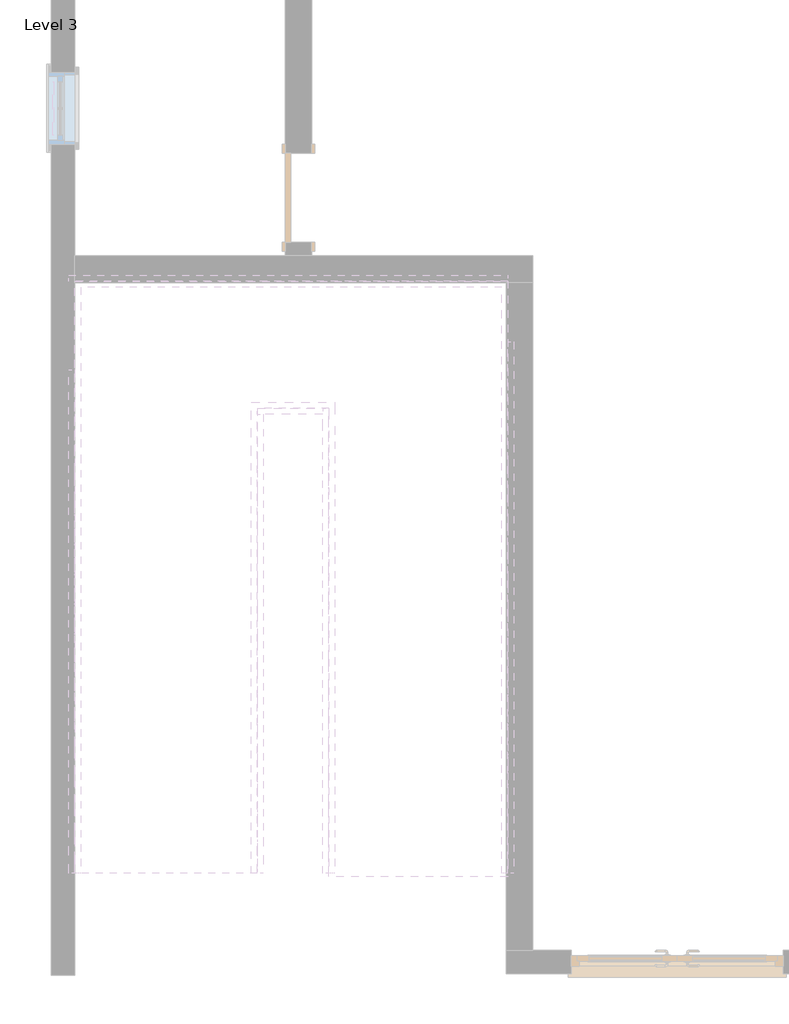
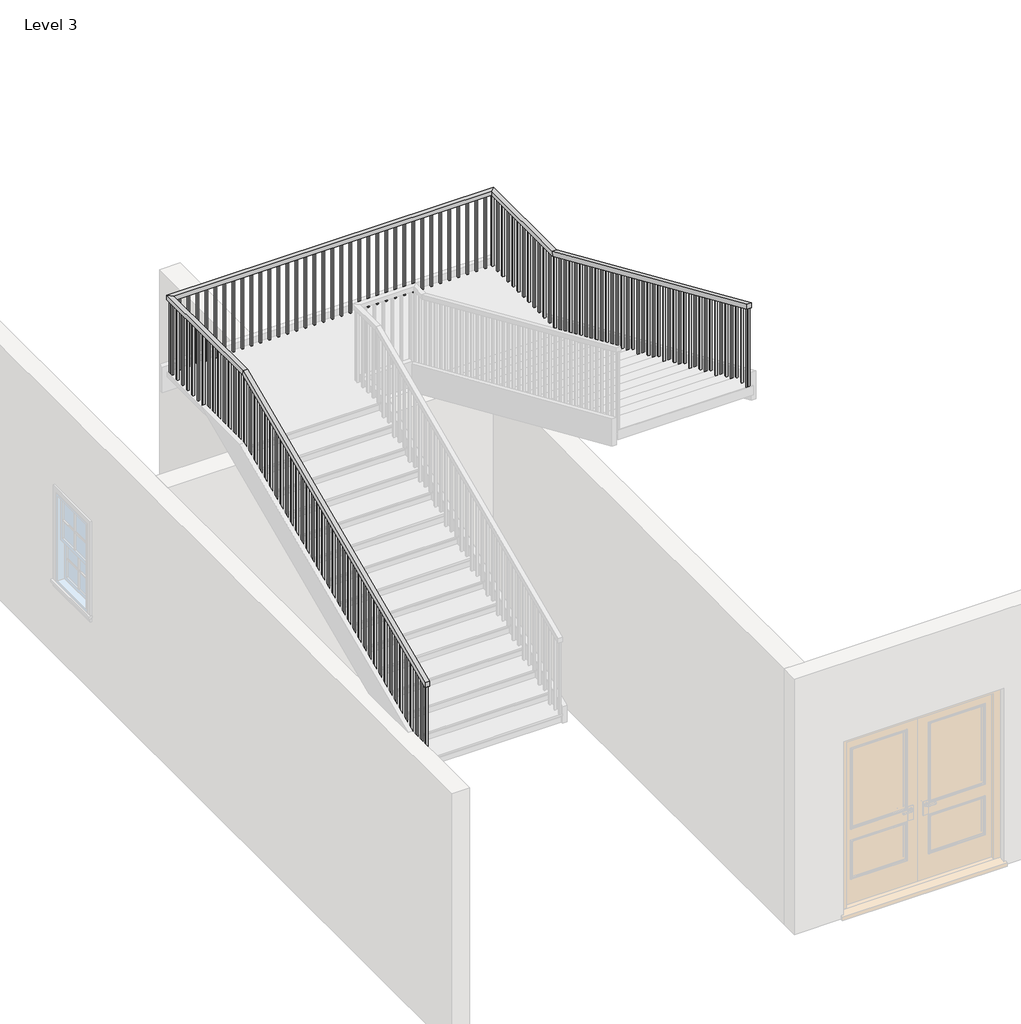
# One storey, part 3 of 6: 1 railing.
"""IFC4 building model written with IfcOpenShell, lengths in millimetres."""

from ifc_helpers import new_model, si_unit, frame, origin, place, context, project, spatial, polyline, outline, extrude, faceted_brep, element, save

model = new_model("IFC4")

# Units and contexts
model_context = context("Model", 3, world=origin())
ifc_project = project(units=[si_unit("LENGTHUNIT", "METRE", prefix="MILLI")], contexts=[model_context])

# Site, building, storey
site = spatial("IfcSite", under=ifc_project)
building = spatial("IfcBuilding", under=site)
storey = spatial("IfcBuildingStorey", under=building, Name="Level 3", Elevation=6096.0)

# Railing
placement = place(None, origin())
element("IfcRailing", 1, ObjectType="Handrail - Rectangular", at=placement, inside=storey, context=model_context, shape_type="SolidModel", body=[
    faceted_brep([(-7554.4415084, -6973.0610642, 9865.36), (-7554.4415084, -6973.0610642, 9809.8599828), (-7503.6415084, -6973.0610642, 9809.8599828), (-7503.6415084, -6973.0610642, 9865.36), (-7554.4415084, -3417.0610642, 11430.0), (-7554.4415084, -3406.3792071, 11379.2), (-7503.6415084, -3406.3792071, 11379.2), (-7503.6415084, -3417.0610642, 11430.0), (-7554.4415084, -1928.4217109, 11430.0), (-7554.4415084, -1928.4217109, 11379.2), (-7503.6415084, -1979.2217109, 11379.2), (-7503.6415084, -1979.2217109, 11430.0), (-3866.3290366, -1928.4217109, 11430.0), (-3866.3290366, -1928.4217109, 11379.2), (-3917.1290366, -1979.2217109, 11379.2), (-3917.1290366, -1979.2217109, 11430.0), (-3866.3290366, -3163.0610642, 11430.0), (-3866.3290366, -3173.7429214, 11379.2), (-3917.1290366, -3173.7429214, 11379.2), (-3917.1290366, -3163.0610642, 11430.0), (-3866.3290366, -6973.0610642, 13106.4), (-3917.1290366, -6973.0610642, 13106.4), (-3917.1290366, -6973.0610642, 13050.8999828), (-3866.3290366, -6973.0610642, 13050.8999828)], [[[0, 1, 2, 3]], [[1, 0, 4, 5]], [[2, 1, 5, 6]], [[3, 2, 6, 7]], [[0, 3, 7, 4]], [[5, 4, 8, 9]], [[6, 5, 9, 10]], [[7, 6, 10, 11]], [[4, 7, 11, 8]], [[9, 8, 12, 13]], [[10, 9, 13, 14]], [[11, 10, 14, 15]], [[8, 11, 15, 12]], [[13, 12, 16, 17]], [[14, 13, 17, 18]], [[15, 14, 18, 19]], [[12, 15, 19, 16]], [[20, 21, 22, 23]], [[17, 16, 20, 23]], [[18, 17, 23, 22]], [[19, 18, 22, 21]], [[16, 19, 21, 20]]]),
    extrude(outline(polyline([(-6922.6967109, 13028.7396674), (-6922.6967109, 12080.24), (-6941.7467109, 12080.24), (-6941.7467109, 13037.1216674), (-6922.6967109, 13028.7396674)])), frame((-3901.2540366, 0.0, 0.0), z_axis=(1.0, 0.0, 0.0), x_axis=(0.0, 1.0, 0.0)), (0.0, 0.0, 1.0), 19.05),
    extrude(outline(polyline([(-6821.0967109, 12984.0356674), (-6821.0967109, 12080.24), (-6840.1467109, 12080.24), (-6840.1467109, 12992.4176674), (-6821.0967109, 12984.0356674)])), frame((-3901.2540366, 0.0, 0.0), z_axis=(1.0, 0.0, 0.0), x_axis=(0.0, 1.0, 0.0)), (0.0, 0.0, 1.0), 19.05),
    extrude(outline(polyline([(-6719.4967109, 12939.3316674), (-6719.4967109, 12080.24), (-6738.5467109, 12080.24), (-6738.5467109, 12947.7136674), (-6719.4967109, 12939.3316674)])), frame((-3901.2540366, 0.0, 0.0), z_axis=(1.0, 0.0, 0.0), x_axis=(0.0, 1.0, 0.0)), (0.0, 0.0, 1.0), 19.05),
    extrude(outline(polyline([(-6617.8967109, 12894.6276674), (-6617.8967109, 11968.48), (-6636.9467109, 11968.48), (-6636.9467109, 12903.0096674), (-6617.8967109, 12894.6276674)])), frame((-3901.2540366, 0.0, 0.0), z_axis=(1.0, 0.0, 0.0), x_axis=(0.0, 1.0, 0.0)), (0.0, 0.0, 1.0), 19.05),
    extrude(outline(polyline([(-6516.2967109, 12849.9236674), (-6516.2967109, 11968.48), (-6535.3467109, 11968.48), (-6535.3467109, 12858.3056674), (-6516.2967109, 12849.9236674)])), frame((-3901.2540366, 0.0, 0.0), z_axis=(1.0, 0.0, 0.0), x_axis=(0.0, 1.0, 0.0)), (0.0, 0.0, 1.0), 19.05),
    extrude(outline(polyline([(-6414.6967109, 12805.2196674), (-6414.6967109, 11856.72), (-6433.7467109, 11856.72), (-6433.7467109, 12813.6016674), (-6414.6967109, 12805.2196674)])), frame((-3901.2540366, 0.0, 0.0), z_axis=(1.0, 0.0, 0.0), x_axis=(0.0, 1.0, 0.0)), (0.0, 0.0, 1.0), 19.05),
    extrude(outline(polyline([(-6313.0967109, 12760.5156674), (-6313.0967109, 11856.72), (-6332.1467109, 11856.72), (-6332.1467109, 12768.8976674), (-6313.0967109, 12760.5156674)])), frame((-3901.2540366, 0.0, 0.0), z_axis=(1.0, 0.0, 0.0), x_axis=(0.0, 1.0, 0.0)), (0.0, 0.0, 1.0), 19.05),
    extrude(outline(polyline([(-6211.4967109, 12715.8116674), (-6211.4967109, 11856.72), (-6230.5467109, 11856.72), (-6230.5467109, 12724.1936674), (-6211.4967109, 12715.8116674)])), frame((-3901.2540366, 0.0, 0.0), z_axis=(1.0, 0.0, 0.0), x_axis=(0.0, 1.0, 0.0)), (0.0, 0.0, 1.0), 19.05),
    extrude(outline(polyline([(-6109.8967109, 12671.1076674), (-6109.8967109, 11744.96), (-6128.9467109, 11744.96), (-6128.9467109, 12679.4896674), (-6109.8967109, 12671.1076674)])), frame((-3901.2540366, 0.0, 0.0), z_axis=(1.0, 0.0, 0.0), x_axis=(0.0, 1.0, 0.0)), (0.0, 0.0, 1.0), 19.05),
    extrude(outline(polyline([(-6008.2967109, 12626.4036674), (-6008.2967109, 11744.96), (-6027.3467109, 11744.96), (-6027.3467109, 12634.7856674), (-6008.2967109, 12626.4036674)])), frame((-3901.2540366, 0.0, 0.0), z_axis=(1.0, 0.0, 0.0), x_axis=(0.0, 1.0, 0.0)), (0.0, 0.0, 1.0), 19.05),
    extrude(outline(polyline([(-5906.6967109, 12581.6996674), (-5906.6967109, 11633.2), (-5925.7467109, 11633.2), (-5925.7467109, 12590.0816674), (-5906.6967109, 12581.6996674)])), frame((-3901.2540366, 0.0, 0.0), z_axis=(1.0, 0.0, 0.0), x_axis=(0.0, 1.0, 0.0)), (0.0, 0.0, 1.0), 19.05),
    extrude(outline(polyline([(-5805.0967109, 12536.9956674), (-5805.0967109, 11633.2), (-5824.1467109, 11633.2), (-5824.1467109, 12545.3776674), (-5805.0967109, 12536.9956674)])), frame((-3901.2540366, 0.0, 0.0), z_axis=(1.0, 0.0, 0.0), x_axis=(0.0, 1.0, 0.0)), (0.0, 0.0, 1.0), 19.05),
    extrude(outline(polyline([(-5703.4967109, 12492.2916674), (-5703.4967109, 11633.2), (-5722.5467109, 11633.2), (-5722.5467109, 12500.6736674), (-5703.4967109, 12492.2916674)])), frame((-3901.2540366, 0.0, 0.0), z_axis=(1.0, 0.0, 0.0), x_axis=(0.0, 1.0, 0.0)), (0.0, 0.0, 1.0), 19.05),
    extrude(outline(polyline([(-5601.8967109, 12447.5876674), (-5601.8967109, 11521.44), (-5620.9467109, 11521.44), (-5620.9467109, 12455.9696674), (-5601.8967109, 12447.5876674)])), frame((-3901.2540366, 0.0, 0.0), z_axis=(1.0, 0.0, 0.0), x_axis=(0.0, 1.0, 0.0)), (0.0, 0.0, 1.0), 19.05),
    extrude(outline(polyline([(-5500.2967109, 12402.8836674), (-5500.2967109, 11521.44), (-5519.3467109, 11521.44), (-5519.3467109, 12411.2656674), (-5500.2967109, 12402.8836674)])), frame((-3901.2540366, 0.0, 0.0), z_axis=(1.0, 0.0, 0.0), x_axis=(0.0, 1.0, 0.0)), (0.0, 0.0, 1.0), 19.05),
    extrude(outline(polyline([(-5398.6967109, 12358.1796674), (-5398.6967109, 11409.68), (-5417.7467109, 11409.68), (-5417.7467109, 12366.5616674), (-5398.6967109, 12358.1796674)])), frame((-3901.2540366, 0.0, 0.0), z_axis=(1.0, 0.0, 0.0), x_axis=(0.0, 1.0, 0.0)), (0.0, 0.0, 1.0), 19.05),
    extrude(outline(polyline([(-5297.0967109, 12313.4756674), (-5297.0967109, 11409.68), (-5316.1467109, 11409.68), (-5316.1467109, 12321.8576674), (-5297.0967109, 12313.4756674)])), frame((-3901.2540366, 0.0, 0.0), z_axis=(1.0, 0.0, 0.0), x_axis=(0.0, 1.0, 0.0)), (0.0, 0.0, 1.0), 19.05),
    extrude(outline(polyline([(-5195.4967109, 12268.7716674), (-5195.4967109, 11409.68), (-5214.5467109, 11409.68), (-5214.5467109, 12277.1536674), (-5195.4967109, 12268.7716674)])), frame((-3901.2540366, 0.0, 0.0), z_axis=(1.0, 0.0, 0.0), x_axis=(0.0, 1.0, 0.0)), (0.0, 0.0, 1.0), 19.05),
    extrude(outline(polyline([(-5093.8967109, 12224.0676674), (-5093.8967109, 11297.92), (-5112.9467109, 11297.92), (-5112.9467109, 12232.4496674), (-5093.8967109, 12224.0676674)])), frame((-3901.2540366, 0.0, 0.0), z_axis=(1.0, 0.0, 0.0), x_axis=(0.0, 1.0, 0.0)), (0.0, 0.0, 1.0), 19.05),
    extrude(outline(polyline([(-4992.2967109, 12179.3636674), (-4992.2967109, 11297.92), (-5011.3467109, 11297.92), (-5011.3467109, 12187.7456674), (-4992.2967109, 12179.3636674)])), frame((-3901.2540366, 0.0, 0.0), z_axis=(1.0, 0.0, 0.0), x_axis=(0.0, 1.0, 0.0)), (0.0, 0.0, 1.0), 19.05),
    extrude(outline(polyline([(-4890.6967109, 12134.6596674), (-4890.6967109, 11186.16), (-4909.7467109, 11186.16), (-4909.7467109, 12143.0416674), (-4890.6967109, 12134.6596674)])), frame((-3901.2540366, 0.0, 0.0), z_axis=(1.0, 0.0, 0.0), x_axis=(0.0, 1.0, 0.0)), (0.0, 0.0, 1.0), 19.05),
    extrude(outline(polyline([(-4789.0967109, 12089.9556674), (-4789.0967109, 11186.16), (-4808.1467109, 11186.16), (-4808.1467109, 12098.3376674), (-4789.0967109, 12089.9556674)])), frame((-3901.2540366, 0.0, 0.0), z_axis=(1.0, 0.0, 0.0), x_axis=(0.0, 1.0, 0.0)), (0.0, 0.0, 1.0), 19.05),
    extrude(outline(polyline([(-4687.4967109, 12045.2516674), (-4687.4967109, 11186.16), (-4706.5467109, 11186.16), (-4706.5467109, 12053.6336674), (-4687.4967109, 12045.2516674)])), frame((-3901.2540366, 0.0, 0.0), z_axis=(1.0, 0.0, 0.0), x_axis=(0.0, 1.0, 0.0)), (0.0, 0.0, 1.0), 19.05),
    extrude(outline(polyline([(-4585.8967109, 12000.5476674), (-4585.8967109, 11074.4), (-4604.9467109, 11074.4), (-4604.9467109, 12008.9296674), (-4585.8967109, 12000.5476674)])), frame((-3901.2540366, 0.0, 0.0), z_axis=(1.0, 0.0, 0.0), x_axis=(0.0, 1.0, 0.0)), (0.0, 0.0, 1.0), 19.05),
    extrude(outline(polyline([(-4484.2967109, 11955.8436674), (-4484.2967109, 11074.4), (-4503.3467109, 11074.4), (-4503.3467109, 11964.2256674), (-4484.2967109, 11955.8436674)])), frame((-3901.2540366, 0.0, 0.0), z_axis=(1.0, 0.0, 0.0), x_axis=(0.0, 1.0, 0.0)), (0.0, 0.0, 1.0), 19.05),
    extrude(outline(polyline([(-4382.6967109, 11911.1396674), (-4382.6967109, 10962.64), (-4401.7467109, 10962.64), (-4401.7467109, 11919.5216674), (-4382.6967109, 11911.1396674)])), frame((-3901.2540366, 0.0, 0.0), z_axis=(1.0, 0.0, 0.0), x_axis=(0.0, 1.0, 0.0)), (0.0, 0.0, 1.0), 19.05),
    extrude(outline(polyline([(-4281.0967109, 11866.4356674), (-4281.0967109, 10962.64), (-4300.1467109, 10962.64), (-4300.1467109, 11874.8176674), (-4281.0967109, 11866.4356674)])), frame((-3901.2540366, 0.0, 0.0), z_axis=(1.0, 0.0, 0.0), x_axis=(0.0, 1.0, 0.0)), (0.0, 0.0, 1.0), 19.05),
    extrude(outline(polyline([(-4179.4967109, 11821.7316674), (-4179.4967109, 10962.64), (-4198.5467109, 10962.64), (-4198.5467109, 11830.1136674), (-4179.4967109, 11821.7316674)])), frame((-3901.2540366, 0.0, 0.0), z_axis=(1.0, 0.0, 0.0), x_axis=(0.0, 1.0, 0.0)), (0.0, 0.0, 1.0), 19.05),
    extrude(outline(polyline([(-4077.8967109, 11777.0276674), (-4077.8967109, 10850.88), (-4096.9467109, 10850.88), (-4096.9467109, 11785.4096674), (-4077.8967109, 11777.0276674)])), frame((-3901.2540366, 0.0, 0.0), z_axis=(1.0, 0.0, 0.0), x_axis=(0.0, 1.0, 0.0)), (0.0, 0.0, 1.0), 19.05),
    extrude(outline(polyline([(-3976.2967109, 11732.3236674), (-3976.2967109, 10850.88), (-3995.3467109, 10850.88), (-3995.3467109, 11740.7056674), (-3976.2967109, 11732.3236674)])), frame((-3901.2540366, 0.0, 0.0), z_axis=(1.0, 0.0, 0.0), x_axis=(0.0, 1.0, 0.0)), (0.0, 0.0, 1.0), 19.05),
    extrude(outline(polyline([(-3874.6967109, 11687.6196674), (-3874.6967109, 10739.12), (-3893.7467109, 10739.12), (-3893.7467109, 11696.0016674), (-3874.6967109, 11687.6196674)])), frame((-3901.2540366, 0.0, 0.0), z_axis=(1.0, 0.0, 0.0), x_axis=(0.0, 1.0, 0.0)), (0.0, 0.0, 1.0), 19.05),
    extrude(outline(polyline([(-3773.0967109, 11642.9156674), (-3773.0967109, 10739.12), (-3792.1467109, 10739.12), (-3792.1467109, 11651.2976674), (-3773.0967109, 11642.9156674)])), frame((-3901.2540366, 0.0, 0.0), z_axis=(1.0, 0.0, 0.0), x_axis=(0.0, 1.0, 0.0)), (0.0, 0.0, 1.0), 19.05),
    extrude(outline(polyline([(-3671.4967109, 11598.2116674), (-3671.4967109, 10739.12), (-3690.5467109, 10739.12), (-3690.5467109, 11606.5936674), (-3671.4967109, 11598.2116674)])), frame((-3901.2540366, 0.0, 0.0), z_axis=(1.0, 0.0, 0.0), x_axis=(0.0, 1.0, 0.0)), (0.0, 0.0, 1.0), 19.05),
    extrude(outline(polyline([(-3569.8967109, 11553.5076674), (-3569.8967109, 10627.36), (-3588.9467109, 10627.36), (-3588.9467109, 11561.8896674), (-3569.8967109, 11553.5076674)])), frame((-3901.2540366, 0.0, 0.0), z_axis=(1.0, 0.0, 0.0), x_axis=(0.0, 1.0, 0.0)), (0.0, 0.0, 1.0), 19.05),
    extrude(outline(polyline([(-3468.2967109, 11508.8036674), (-3468.2967109, 10627.36), (-3487.3467109, 10627.36), (-3487.3467109, 11517.1856674), (-3468.2967109, 11508.8036674)])), frame((-3901.2540366, 0.0, 0.0), z_axis=(1.0, 0.0, 0.0), x_axis=(0.0, 1.0, 0.0)), (0.0, 0.0, 1.0), 19.05),
    extrude(outline(polyline([(-3366.6967109, 11464.0996674), (-3366.6967109, 10515.6), (-3385.7467109, 10515.6), (-3385.7467109, 11472.4816674), (-3366.6967109, 11464.0996674)])), frame((-3901.2540366, 0.0, 0.0), z_axis=(1.0, 0.0, 0.0), x_axis=(0.0, 1.0, 0.0)), (0.0, 0.0, 1.0), 19.05),
    extrude(outline(polyline([(-3265.0967109, 11419.3956674), (-3265.0967109, 10515.6), (-3284.1467109, 10515.6), (-3284.1467109, 11427.7776674), (-3265.0967109, 11419.3956674)])), frame((-3901.2540366, 0.0, 0.0), z_axis=(1.0, 0.0, 0.0), x_axis=(0.0, 1.0, 0.0)), (0.0, 0.0, 1.0), 19.05),
    extrude(outline(polyline([(-3163.4967109, 11374.6916674), (-3163.4967109, 10515.6), (-3182.5467109, 10515.6), (-3182.5467109, 11383.0736674), (-3163.4967109, 11374.6916674)])), frame((-3901.2540366, 0.0, 0.0), z_axis=(1.0, 0.0, 0.0), x_axis=(0.0, 1.0, 0.0)), (0.0, 0.0, 1.0), 19.05),
    extrude(outline(polyline([(-3882.2040366, -3061.8967109), (-3882.2040366, -3080.9467109), (-3901.2540366, -3080.9467109), (-3901.2540366, -3061.8967109), (-3882.2040366, -3061.8967109)])), frame((0.0, 0.0, 10515.6), z_axis=(0.0, 0.0, 1.0), x_axis=(1.0, 0.0, 0.0)), (0.0, 0.0, 1.0), 863.6),
    extrude(outline(polyline([(-3882.2040366, -2960.2967109), (-3882.2040366, -2979.3467109), (-3901.2540366, -2979.3467109), (-3901.2540366, -2960.2967109), (-3882.2040366, -2960.2967109)])), frame((0.0, 0.0, 10515.6), z_axis=(0.0, 0.0, 1.0), x_axis=(1.0, 0.0, 0.0)), (0.0, 0.0, 1.0), 863.6),
    extrude(outline(polyline([(-3882.2040366, -2858.6967109), (-3882.2040366, -2877.7467109), (-3901.2540366, -2877.7467109), (-3901.2540366, -2858.6967109), (-3882.2040366, -2858.6967109)])), frame((0.0, 0.0, 10515.6), z_axis=(0.0, 0.0, 1.0), x_axis=(1.0, 0.0, 0.0)), (0.0, 0.0, 1.0), 863.6),
    extrude(outline(polyline([(-3882.2040366, -2757.0967109), (-3882.2040366, -2776.1467109), (-3901.2540366, -2776.1467109), (-3901.2540366, -2757.0967109), (-3882.2040366, -2757.0967109)])), frame((0.0, 0.0, 10515.6), z_axis=(0.0, 0.0, 1.0), x_axis=(1.0, 0.0, 0.0)), (0.0, 0.0, 1.0), 863.6),
    extrude(outline(polyline([(-3882.2040366, -2655.4967109), (-3882.2040366, -2674.5467109), (-3901.2540366, -2674.5467109), (-3901.2540366, -2655.4967109), (-3882.2040366, -2655.4967109)])), frame((0.0, 0.0, 10515.6), z_axis=(0.0, 0.0, 1.0), x_axis=(1.0, 0.0, 0.0)), (0.0, 0.0, 1.0), 863.6),
    extrude(outline(polyline([(-3882.2040366, -2553.8967109), (-3882.2040366, -2572.9467109), (-3901.2540366, -2572.9467109), (-3901.2540366, -2553.8967109), (-3882.2040366, -2553.8967109)])), frame((0.0, 0.0, 10515.6), z_axis=(0.0, 0.0, 1.0), x_axis=(1.0, 0.0, 0.0)), (0.0, 0.0, 1.0), 863.6),
    extrude(outline(polyline([(-3882.2040366, -2452.2967109), (-3882.2040366, -2471.3467109), (-3901.2540366, -2471.3467109), (-3901.2540366, -2452.2967109), (-3882.2040366, -2452.2967109)])), frame((0.0, 0.0, 10515.6), z_axis=(0.0, 0.0, 1.0), x_axis=(1.0, 0.0, 0.0)), (0.0, 0.0, 1.0), 863.6),
    extrude(outline(polyline([(-3882.2040366, -2350.6967109), (-3882.2040366, -2369.7467109), (-3901.2540366, -2369.7467109), (-3901.2540366, -2350.6967109), (-3882.2040366, -2350.6967109)])), frame((0.0, 0.0, 10515.6), z_axis=(0.0, 0.0, 1.0), x_axis=(1.0, 0.0, 0.0)), (0.0, 0.0, 1.0), 863.6),
    extrude(outline(polyline([(-3882.2040366, -2249.0967109), (-3882.2040366, -2268.1467109), (-3901.2540366, -2268.1467109), (-3901.2540366, -2249.0967109), (-3882.2040366, -2249.0967109)])), frame((0.0, 0.0, 10515.6), z_axis=(0.0, 0.0, 1.0), x_axis=(1.0, 0.0, 0.0)), (0.0, 0.0, 1.0), 863.6),
    extrude(outline(polyline([(-3882.2040366, -2147.4967109), (-3882.2040366, -2166.5467109), (-3901.2540366, -2166.5467109), (-3901.2540366, -2147.4967109), (-3882.2040366, -2147.4967109)])), frame((0.0, 0.0, 10515.6), z_axis=(0.0, 0.0, 1.0), x_axis=(1.0, 0.0, 0.0)), (0.0, 0.0, 1.0), 863.6),
    extrude(outline(polyline([(-3882.2040366, -2045.8967109), (-3882.2040366, -2064.9467109), (-3901.2540366, -2064.9467109), (-3901.2540366, -2045.8967109), (-3882.2040366, -2045.8967109)])), frame((0.0, 0.0, 10515.6), z_axis=(0.0, 0.0, 1.0), x_axis=(1.0, 0.0, 0.0)), (0.0, 0.0, 1.0), 863.6),
    extrude(outline(polyline([(-3982.5665084, -1944.2967109), (-3963.5165084, -1944.2967109), (-3963.5165084, -1963.3467109), (-3982.5665084, -1963.3467109), (-3982.5665084, -1944.2967109)])), frame((0.0, 0.0, 10515.6), z_axis=(0.0, 0.0, 1.0), x_axis=(1.0, 0.0, 0.0)), (0.0, 0.0, 1.0), 863.6),
    extrude(outline(polyline([(-4084.1665084, -1944.2967109), (-4065.1165084, -1944.2967109), (-4065.1165084, -1963.3467109), (-4084.1665084, -1963.3467109), (-4084.1665084, -1944.2967109)])), frame((0.0, 0.0, 10515.6), z_axis=(0.0, 0.0, 1.0), x_axis=(1.0, 0.0, 0.0)), (0.0, 0.0, 1.0), 863.6),
    extrude(outline(polyline([(-4185.7665084, -1944.2967109), (-4166.7165084, -1944.2967109), (-4166.7165084, -1963.3467109), (-4185.7665084, -1963.3467109), (-4185.7665084, -1944.2967109)])), frame((0.0, 0.0, 10515.6), z_axis=(0.0, 0.0, 1.0), x_axis=(1.0, 0.0, 0.0)), (0.0, 0.0, 1.0), 863.6),
    extrude(outline(polyline([(-4287.3665084, -1944.2967109), (-4268.3165084, -1944.2967109), (-4268.3165084, -1963.3467109), (-4287.3665084, -1963.3467109), (-4287.3665084, -1944.2967109)])), frame((0.0, 0.0, 10515.6), z_axis=(0.0, 0.0, 1.0), x_axis=(1.0, 0.0, 0.0)), (0.0, 0.0, 1.0), 863.6),
    extrude(outline(polyline([(-4388.9665084, -1944.2967109), (-4369.9165084, -1944.2967109), (-4369.9165084, -1963.3467109), (-4388.9665084, -1963.3467109), (-4388.9665084, -1944.2967109)])), frame((0.0, 0.0, 10515.6), z_axis=(0.0, 0.0, 1.0), x_axis=(1.0, 0.0, 0.0)), (0.0, 0.0, 1.0), 863.6),
    extrude(outline(polyline([(-4490.5665084, -1944.2967109), (-4471.5165084, -1944.2967109), (-4471.5165084, -1963.3467109), (-4490.5665084, -1963.3467109), (-4490.5665084, -1944.2967109)])), frame((0.0, 0.0, 10515.6), z_axis=(0.0, 0.0, 1.0), x_axis=(1.0, 0.0, 0.0)), (0.0, 0.0, 1.0), 863.6),
    extrude(outline(polyline([(-4592.1665084, -1944.2967109), (-4573.1165084, -1944.2967109), (-4573.1165084, -1963.3467109), (-4592.1665084, -1963.3467109), (-4592.1665084, -1944.2967109)])), frame((0.0, 0.0, 10515.6), z_axis=(0.0, 0.0, 1.0), x_axis=(1.0, 0.0, 0.0)), (0.0, 0.0, 1.0), 863.6),
    extrude(outline(polyline([(-4693.7665084, -1944.2967109), (-4674.7165084, -1944.2967109), (-4674.7165084, -1963.3467109), (-4693.7665084, -1963.3467109), (-4693.7665084, -1944.2967109)])), frame((0.0, 0.0, 10515.6), z_axis=(0.0, 0.0, 1.0), x_axis=(1.0, 0.0, 0.0)), (0.0, 0.0, 1.0), 863.6),
    extrude(outline(polyline([(-4795.3665084, -1944.2967109), (-4776.3165084, -1944.2967109), (-4776.3165084, -1963.3467109), (-4795.3665084, -1963.3467109), (-4795.3665084, -1944.2967109)])), frame((0.0, 0.0, 10515.6), z_axis=(0.0, 0.0, 1.0), x_axis=(1.0, 0.0, 0.0)), (0.0, 0.0, 1.0), 863.6),
    extrude(outline(polyline([(-4896.9665084, -1944.2967109), (-4877.9165084, -1944.2967109), (-4877.9165084, -1963.3467109), (-4896.9665084, -1963.3467109), (-4896.9665084, -1944.2967109)])), frame((0.0, 0.0, 10515.6), z_axis=(0.0, 0.0, 1.0), x_axis=(1.0, 0.0, 0.0)), (0.0, 0.0, 1.0), 863.6),
    extrude(outline(polyline([(-4998.5665084, -1944.2967109), (-4979.5165084, -1944.2967109), (-4979.5165084, -1963.3467109), (-4998.5665084, -1963.3467109), (-4998.5665084, -1944.2967109)])), frame((0.0, 0.0, 10515.6), z_axis=(0.0, 0.0, 1.0), x_axis=(1.0, 0.0, 0.0)), (0.0, 0.0, 1.0), 863.6),
    extrude(outline(polyline([(-5100.1665084, -1944.2967109), (-5081.1165084, -1944.2967109), (-5081.1165084, -1963.3467109), (-5100.1665084, -1963.3467109), (-5100.1665084, -1944.2967109)])), frame((0.0, 0.0, 10515.6), z_axis=(0.0, 0.0, 1.0), x_axis=(1.0, 0.0, 0.0)), (0.0, 0.0, 1.0), 863.6),
    extrude(outline(polyline([(-5201.7665084, -1944.2967109), (-5182.7165084, -1944.2967109), (-5182.7165084, -1963.3467109), (-5201.7665084, -1963.3467109), (-5201.7665084, -1944.2967109)])), frame((0.0, 0.0, 10515.6), z_axis=(0.0, 0.0, 1.0), x_axis=(1.0, 0.0, 0.0)), (0.0, 0.0, 1.0), 863.6),
    extrude(outline(polyline([(-5303.3665084, -1944.2967109), (-5284.3165084, -1944.2967109), (-5284.3165084, -1963.3467109), (-5303.3665084, -1963.3467109), (-5303.3665084, -1944.2967109)])), frame((0.0, 0.0, 10515.6), z_axis=(0.0, 0.0, 1.0), x_axis=(1.0, 0.0, 0.0)), (0.0, 0.0, 1.0), 863.6),
    extrude(outline(polyline([(-5404.9665084, -1944.2967109), (-5385.9165084, -1944.2967109), (-5385.9165084, -1963.3467109), (-5404.9665084, -1963.3467109), (-5404.9665084, -1944.2967109)])), frame((0.0, 0.0, 10515.6), z_axis=(0.0, 0.0, 1.0), x_axis=(1.0, 0.0, 0.0)), (0.0, 0.0, 1.0), 863.6),
    extrude(outline(polyline([(-5506.5665084, -1944.2967109), (-5487.5165084, -1944.2967109), (-5487.5165084, -1963.3467109), (-5506.5665084, -1963.3467109), (-5506.5665084, -1944.2967109)])), frame((0.0, 0.0, 10515.6), z_axis=(0.0, 0.0, 1.0), x_axis=(1.0, 0.0, 0.0)), (0.0, 0.0, 1.0), 863.6),
    extrude(outline(polyline([(-5608.1665084, -1944.2967109), (-5589.1165084, -1944.2967109), (-5589.1165084, -1963.3467109), (-5608.1665084, -1963.3467109), (-5608.1665084, -1944.2967109)])), frame((0.0, 0.0, 10515.6), z_axis=(0.0, 0.0, 1.0), x_axis=(1.0, 0.0, 0.0)), (0.0, 0.0, 1.0), 863.6),
    extrude(outline(polyline([(-5709.7665084, -1944.2967109), (-5690.7165084, -1944.2967109), (-5690.7165084, -1963.3467109), (-5709.7665084, -1963.3467109), (-5709.7665084, -1944.2967109)])), frame((0.0, 0.0, 10515.6), z_axis=(0.0, 0.0, 1.0), x_axis=(1.0, 0.0, 0.0)), (0.0, 0.0, 1.0), 863.6),
    extrude(outline(polyline([(-5811.3665084, -1944.2967109), (-5792.3165084, -1944.2967109), (-5792.3165084, -1963.3467109), (-5811.3665084, -1963.3467109), (-5811.3665084, -1944.2967109)])), frame((0.0, 0.0, 10515.6), z_axis=(0.0, 0.0, 1.0), x_axis=(1.0, 0.0, 0.0)), (0.0, 0.0, 1.0), 863.6),
    extrude(outline(polyline([(-5912.9665084, -1944.2967109), (-5893.9165084, -1944.2967109), (-5893.9165084, -1963.3467109), (-5912.9665084, -1963.3467109), (-5912.9665084, -1944.2967109)])), frame((0.0, 0.0, 10515.6), z_axis=(0.0, 0.0, 1.0), x_axis=(1.0, 0.0, 0.0)), (0.0, 0.0, 1.0), 863.6),
    extrude(outline(polyline([(-6014.5665084, -1944.2967109), (-5995.5165084, -1944.2967109), (-5995.5165084, -1963.3467109), (-6014.5665084, -1963.3467109), (-6014.5665084, -1944.2967109)])), frame((0.0, 0.0, 10515.6), z_axis=(0.0, 0.0, 1.0), x_axis=(1.0, 0.0, 0.0)), (0.0, 0.0, 1.0), 863.6),
    extrude(outline(polyline([(-6116.1665084, -1944.2967109), (-6097.1165084, -1944.2967109), (-6097.1165084, -1963.3467109), (-6116.1665084, -1963.3467109), (-6116.1665084, -1944.2967109)])), frame((0.0, 0.0, 10515.6), z_axis=(0.0, 0.0, 1.0), x_axis=(1.0, 0.0, 0.0)), (0.0, 0.0, 1.0), 863.6),
    extrude(outline(polyline([(-6217.7665084, -1944.2967109), (-6198.7165084, -1944.2967109), (-6198.7165084, -1963.3467109), (-6217.7665084, -1963.3467109), (-6217.7665084, -1944.2967109)])), frame((0.0, 0.0, 10515.6), z_axis=(0.0, 0.0, 1.0), x_axis=(1.0, 0.0, 0.0)), (0.0, 0.0, 1.0), 863.6),
    extrude(outline(polyline([(-6319.3665084, -1944.2967109), (-6300.3165084, -1944.2967109), (-6300.3165084, -1963.3467109), (-6319.3665084, -1963.3467109), (-6319.3665084, -1944.2967109)])), frame((0.0, 0.0, 10515.6), z_axis=(0.0, 0.0, 1.0), x_axis=(1.0, 0.0, 0.0)), (0.0, 0.0, 1.0), 863.6),
    extrude(outline(polyline([(-6420.9665084, -1944.2967109), (-6401.9165084, -1944.2967109), (-6401.9165084, -1963.3467109), (-6420.9665084, -1963.3467109), (-6420.9665084, -1944.2967109)])), frame((0.0, 0.0, 10515.6), z_axis=(0.0, 0.0, 1.0), x_axis=(1.0, 0.0, 0.0)), (0.0, 0.0, 1.0), 863.6),
    extrude(outline(polyline([(-6522.5665084, -1944.2967109), (-6503.5165084, -1944.2967109), (-6503.5165084, -1963.3467109), (-6522.5665084, -1963.3467109), (-6522.5665084, -1944.2967109)])), frame((0.0, 0.0, 10515.6), z_axis=(0.0, 0.0, 1.0), x_axis=(1.0, 0.0, 0.0)), (0.0, 0.0, 1.0), 863.6),
    extrude(outline(polyline([(-6624.1665084, -1944.2967109), (-6605.1165084, -1944.2967109), (-6605.1165084, -1963.3467109), (-6624.1665084, -1963.3467109), (-6624.1665084, -1944.2967109)])), frame((0.0, 0.0, 10515.6), z_axis=(0.0, 0.0, 1.0), x_axis=(1.0, 0.0, 0.0)), (0.0, 0.0, 1.0), 863.6),
    extrude(outline(polyline([(-6725.7665084, -1944.2967109), (-6706.7165084, -1944.2967109), (-6706.7165084, -1963.3467109), (-6725.7665084, -1963.3467109), (-6725.7665084, -1944.2967109)])), frame((0.0, 0.0, 10515.6), z_axis=(0.0, 0.0, 1.0), x_axis=(1.0, 0.0, 0.0)), (0.0, 0.0, 1.0), 863.6),
    extrude(outline(polyline([(-6827.3665084, -1944.2967109), (-6808.3165084, -1944.2967109), (-6808.3165084, -1963.3467109), (-6827.3665084, -1963.3467109), (-6827.3665084, -1944.2967109)])), frame((0.0, 0.0, 10515.6), z_axis=(0.0, 0.0, 1.0), x_axis=(1.0, 0.0, 0.0)), (0.0, 0.0, 1.0), 863.6),
    extrude(outline(polyline([(-6928.9665084, -1944.2967109), (-6909.9165084, -1944.2967109), (-6909.9165084, -1963.3467109), (-6928.9665084, -1963.3467109), (-6928.9665084, -1944.2967109)])), frame((0.0, 0.0, 10515.6), z_axis=(0.0, 0.0, 1.0), x_axis=(1.0, 0.0, 0.0)), (0.0, 0.0, 1.0), 863.6),
    extrude(outline(polyline([(-7030.5665084, -1944.2967109), (-7011.5165084, -1944.2967109), (-7011.5165084, -1963.3467109), (-7030.5665084, -1963.3467109), (-7030.5665084, -1944.2967109)])), frame((0.0, 0.0, 10515.6), z_axis=(0.0, 0.0, 1.0), x_axis=(1.0, 0.0, 0.0)), (0.0, 0.0, 1.0), 863.6),
    extrude(outline(polyline([(-7132.1665084, -1944.2967109), (-7113.1165084, -1944.2967109), (-7113.1165084, -1963.3467109), (-7132.1665084, -1963.3467109), (-7132.1665084, -1944.2967109)])), frame((0.0, 0.0, 10515.6), z_axis=(0.0, 0.0, 1.0), x_axis=(1.0, 0.0, 0.0)), (0.0, 0.0, 1.0), 863.6),
    extrude(outline(polyline([(-7233.7665084, -1944.2967109), (-7214.7165084, -1944.2967109), (-7214.7165084, -1963.3467109), (-7233.7665084, -1963.3467109), (-7233.7665084, -1944.2967109)])), frame((0.0, 0.0, 10515.6), z_axis=(0.0, 0.0, 1.0), x_axis=(1.0, 0.0, 0.0)), (0.0, 0.0, 1.0), 863.6),
    extrude(outline(polyline([(-7335.3665084, -1944.2967109), (-7316.3165084, -1944.2967109), (-7316.3165084, -1963.3467109), (-7335.3665084, -1963.3467109), (-7335.3665084, -1944.2967109)])), frame((0.0, 0.0, 10515.6), z_axis=(0.0, 0.0, 1.0), x_axis=(1.0, 0.0, 0.0)), (0.0, 0.0, 1.0), 863.6),
    extrude(outline(polyline([(-7436.9665084, -1944.2967109), (-7417.9165084, -1944.2967109), (-7417.9165084, -1963.3467109), (-7436.9665084, -1963.3467109), (-7436.9665084, -1944.2967109)])), frame((0.0, 0.0, 10515.6), z_axis=(0.0, 0.0, 1.0), x_axis=(1.0, 0.0, 0.0)), (0.0, 0.0, 1.0), 863.6),
    extrude(outline(polyline([(-7538.5665084, -2004.1860642), (-7538.5665084, -1985.1360642), (-7519.5165084, -1985.1360642), (-7519.5165084, -2004.1860642), (-7538.5665084, -2004.1860642)])), frame((0.0, 0.0, 10515.6), z_axis=(0.0, 0.0, 1.0), x_axis=(1.0, 0.0, 0.0)), (0.0, 0.0, 1.0), 863.6),
    extrude(outline(polyline([(-7538.5665084, -2105.7860642), (-7538.5665084, -2086.7360642), (-7519.5165084, -2086.7360642), (-7519.5165084, -2105.7860642), (-7538.5665084, -2105.7860642)])), frame((0.0, 0.0, 10515.6), z_axis=(0.0, 0.0, 1.0), x_axis=(1.0, 0.0, 0.0)), (0.0, 0.0, 1.0), 863.6),
    extrude(outline(polyline([(-7538.5665084, -2207.3860642), (-7538.5665084, -2188.3360642), (-7519.5165084, -2188.3360642), (-7519.5165084, -2207.3860642), (-7538.5665084, -2207.3860642)])), frame((0.0, 0.0, 10515.6), z_axis=(0.0, 0.0, 1.0), x_axis=(1.0, 0.0, 0.0)), (0.0, 0.0, 1.0), 863.6),
    extrude(outline(polyline([(-7538.5665084, -2308.9860642), (-7538.5665084, -2289.9360642), (-7519.5165084, -2289.9360642), (-7519.5165084, -2308.9860642), (-7538.5665084, -2308.9860642)])), frame((0.0, 0.0, 10515.6), z_axis=(0.0, 0.0, 1.0), x_axis=(1.0, 0.0, 0.0)), (0.0, 0.0, 1.0), 863.6),
    extrude(outline(polyline([(-7538.5665084, -2410.5860642), (-7538.5665084, -2391.5360642), (-7519.5165084, -2391.5360642), (-7519.5165084, -2410.5860642), (-7538.5665084, -2410.5860642)])), frame((0.0, 0.0, 10515.6), z_axis=(0.0, 0.0, 1.0), x_axis=(1.0, 0.0, 0.0)), (0.0, 0.0, 1.0), 863.6),
    extrude(outline(polyline([(-7538.5665084, -2512.1860642), (-7538.5665084, -2493.1360642), (-7519.5165084, -2493.1360642), (-7519.5165084, -2512.1860642), (-7538.5665084, -2512.1860642)])), frame((0.0, 0.0, 10515.6), z_axis=(0.0, 0.0, 1.0), x_axis=(1.0, 0.0, 0.0)), (0.0, 0.0, 1.0), 863.6),
    extrude(outline(polyline([(-7538.5665084, -2613.7860642), (-7538.5665084, -2594.7360642), (-7519.5165084, -2594.7360642), (-7519.5165084, -2613.7860642), (-7538.5665084, -2613.7860642)])), frame((0.0, 0.0, 10515.6), z_axis=(0.0, 0.0, 1.0), x_axis=(1.0, 0.0, 0.0)), (0.0, 0.0, 1.0), 863.6),
    extrude(outline(polyline([(-7538.5665084, -2715.3860642), (-7538.5665084, -2696.3360642), (-7519.5165084, -2696.3360642), (-7519.5165084, -2715.3860642), (-7538.5665084, -2715.3860642)])), frame((0.0, 0.0, 10515.6), z_axis=(0.0, 0.0, 1.0), x_axis=(1.0, 0.0, 0.0)), (0.0, 0.0, 1.0), 863.6),
    extrude(outline(polyline([(-7538.5665084, -2816.9860642), (-7538.5665084, -2797.9360642), (-7519.5165084, -2797.9360642), (-7519.5165084, -2816.9860642), (-7538.5665084, -2816.9860642)])), frame((0.0, 0.0, 10515.6), z_axis=(0.0, 0.0, 1.0), x_axis=(1.0, 0.0, 0.0)), (0.0, 0.0, 1.0), 863.6),
    extrude(outline(polyline([(-7538.5665084, -2918.5860642), (-7538.5665084, -2899.5360642), (-7519.5165084, -2899.5360642), (-7519.5165084, -2918.5860642), (-7538.5665084, -2918.5860642)])), frame((0.0, 0.0, 10515.6), z_axis=(0.0, 0.0, 1.0), x_axis=(1.0, 0.0, 0.0)), (0.0, 0.0, 1.0), 863.6),
    extrude(outline(polyline([(-7538.5665084, -3020.1860642), (-7538.5665084, -3001.1360642), (-7519.5165084, -3001.1360642), (-7519.5165084, -3020.1860642), (-7538.5665084, -3020.1860642)])), frame((0.0, 0.0, 10515.6), z_axis=(0.0, 0.0, 1.0), x_axis=(1.0, 0.0, 0.0)), (0.0, 0.0, 1.0), 863.6),
    extrude(outline(polyline([(-7538.5665084, -3121.7860642), (-7538.5665084, -3102.7360642), (-7519.5165084, -3102.7360642), (-7519.5165084, -3121.7860642), (-7538.5665084, -3121.7860642)])), frame((0.0, 0.0, 10515.6), z_axis=(0.0, 0.0, 1.0), x_axis=(1.0, 0.0, 0.0)), (0.0, 0.0, 1.0), 863.6),
    extrude(outline(polyline([(-7538.5665084, -3223.3860642), (-7538.5665084, -3204.3360642), (-7519.5165084, -3204.3360642), (-7519.5165084, -3223.3860642), (-7538.5665084, -3223.3860642)])), frame((0.0, 0.0, 10515.6), z_axis=(0.0, 0.0, 1.0), x_axis=(1.0, 0.0, 0.0)), (0.0, 0.0, 1.0), 863.6),
    extrude(outline(polyline([(-7538.5665084, -3324.9860642), (-7538.5665084, -3305.9360642), (-7519.5165084, -3305.9360642), (-7519.5165084, -3324.9860642), (-7538.5665084, -3324.9860642)])), frame((0.0, 0.0, 10515.6), z_axis=(0.0, 0.0, 1.0), x_axis=(1.0, 0.0, 0.0)), (0.0, 0.0, 1.0), 863.6),
    extrude(outline(polyline([(-3407.5360642, 11378.6909828), (-3407.5360642, 10515.6), (-3426.5860642, 10515.6), (-3426.5860642, 11370.3089828), (-3407.5360642, 11378.6909828)])), frame((-7538.5665084, 0.0, 0.0), z_axis=(1.0, 0.0, 0.0), x_axis=(0.0, 1.0, 0.0)), (0.0, 0.0, 1.0), 19.05),
    extrude(outline(polyline([(-3509.1360642, 11333.9869828), (-3509.1360642, 10403.84), (-3528.1860642, 10403.84), (-3528.1860642, 11325.6049828), (-3509.1360642, 11333.9869828)])), frame((-7538.5665084, 0.0, 0.0), z_axis=(1.0, 0.0, 0.0), x_axis=(0.0, 1.0, 0.0)), (0.0, 0.0, 1.0), 19.05),
    extrude(outline(polyline([(-3610.7360642, 11289.2829828), (-3610.7360642, 10403.84), (-3629.7860642, 10403.84), (-3629.7860642, 11280.9009828), (-3610.7360642, 11289.2829828)])), frame((-7538.5665084, 0.0, 0.0), z_axis=(1.0, 0.0, 0.0), x_axis=(0.0, 1.0, 0.0)), (0.0, 0.0, 1.0), 19.05),
    extrude(outline(polyline([(-3712.3360642, 11244.5789828), (-3712.3360642, 10292.08), (-3731.3860642, 10292.08), (-3731.3860642, 11236.1969828), (-3712.3360642, 11244.5789828)])), frame((-7538.5665084, 0.0, 0.0), z_axis=(1.0, 0.0, 0.0), x_axis=(0.0, 1.0, 0.0)), (0.0, 0.0, 1.0), 19.05),
    extrude(outline(polyline([(-3813.9360642, 11199.8749828), (-3813.9360642, 10292.08), (-3832.9860642, 10292.08), (-3832.9860642, 11191.4929828), (-3813.9360642, 11199.8749828)])), frame((-7538.5665084, 0.0, 0.0), z_axis=(1.0, 0.0, 0.0), x_axis=(0.0, 1.0, 0.0)), (0.0, 0.0, 1.0), 19.05),
    extrude(outline(polyline([(-3915.5360642, 11155.1709828), (-3915.5360642, 10292.08), (-3934.5860642, 10292.08), (-3934.5860642, 11146.7889828), (-3915.5360642, 11155.1709828)])), frame((-7538.5665084, 0.0, 0.0), z_axis=(1.0, 0.0, 0.0), x_axis=(0.0, 1.0, 0.0)), (0.0, 0.0, 1.0), 19.05),
    extrude(outline(polyline([(-4017.1360642, 11110.4669828), (-4017.1360642, 10180.32), (-4036.1860642, 10180.32), (-4036.1860642, 11102.0849828), (-4017.1360642, 11110.4669828)])), frame((-7538.5665084, 0.0, 0.0), z_axis=(1.0, 0.0, 0.0), x_axis=(0.0, 1.0, 0.0)), (0.0, 0.0, 1.0), 19.05),
    extrude(outline(polyline([(-4118.7360642, 11065.7629828), (-4118.7360642, 10180.32), (-4137.7860642, 10180.32), (-4137.7860642, 11057.3809828), (-4118.7360642, 11065.7629828)])), frame((-7538.5665084, 0.0, 0.0), z_axis=(1.0, 0.0, 0.0), x_axis=(0.0, 1.0, 0.0)), (0.0, 0.0, 1.0), 19.05),
    extrude(outline(polyline([(-4220.3360642, 11021.0589828), (-4220.3360642, 10068.56), (-4239.3860642, 10068.56), (-4239.3860642, 11012.6769828), (-4220.3360642, 11021.0589828)])), frame((-7538.5665084, 0.0, 0.0), z_axis=(1.0, 0.0, 0.0), x_axis=(0.0, 1.0, 0.0)), (0.0, 0.0, 1.0), 19.05),
    extrude(outline(polyline([(-4321.9360642, 10976.3549828), (-4321.9360642, 10068.56), (-4340.9860642, 10068.56), (-4340.9860642, 10967.9729828), (-4321.9360642, 10976.3549828)])), frame((-7538.5665084, 0.0, 0.0), z_axis=(1.0, 0.0, 0.0), x_axis=(0.0, 1.0, 0.0)), (0.0, 0.0, 1.0), 19.05),
    extrude(outline(polyline([(-4423.5360642, 10931.6509828), (-4423.5360642, 10068.56), (-4442.5860642, 10068.56), (-4442.5860642, 10923.2689828), (-4423.5360642, 10931.6509828)])), frame((-7538.5665084, 0.0, 0.0), z_axis=(1.0, 0.0, 0.0), x_axis=(0.0, 1.0, 0.0)), (0.0, 0.0, 1.0), 19.05),
    extrude(outline(polyline([(-4525.1360642, 10886.9469828), (-4525.1360642, 9956.8), (-4544.1860642, 9956.8), (-4544.1860642, 10878.5649828), (-4525.1360642, 10886.9469828)])), frame((-7538.5665084, 0.0, 0.0), z_axis=(1.0, 0.0, 0.0), x_axis=(0.0, 1.0, 0.0)), (0.0, 0.0, 1.0), 19.05),
    extrude(outline(polyline([(-4626.7360642, 10842.2429828), (-4626.7360642, 9956.8), (-4645.7860642, 9956.8), (-4645.7860642, 10833.8609828), (-4626.7360642, 10842.2429828)])), frame((-7538.5665084, 0.0, 0.0), z_axis=(1.0, 0.0, 0.0), x_axis=(0.0, 1.0, 0.0)), (0.0, 0.0, 1.0), 19.05),
    extrude(outline(polyline([(-4728.3360642, 10797.5389828), (-4728.3360642, 9845.04), (-4747.3860642, 9845.04), (-4747.3860642, 10789.1569828), (-4728.3360642, 10797.5389828)])), frame((-7538.5665084, 0.0, 0.0), z_axis=(1.0, 0.0, 0.0), x_axis=(0.0, 1.0, 0.0)), (0.0, 0.0, 1.0), 19.05),
    extrude(outline(polyline([(-4829.9360642, 10752.8349828), (-4829.9360642, 9845.04), (-4848.9860642, 9845.04), (-4848.9860642, 10744.4529828), (-4829.9360642, 10752.8349828)])), frame((-7538.5665084, 0.0, 0.0), z_axis=(1.0, 0.0, 0.0), x_axis=(0.0, 1.0, 0.0)), (0.0, 0.0, 1.0), 19.05),
    extrude(outline(polyline([(-4931.5360642, 10708.1309828), (-4931.5360642, 9845.04), (-4950.5860642, 9845.04), (-4950.5860642, 10699.7489828), (-4931.5360642, 10708.1309828)])), frame((-7538.5665084, 0.0, 0.0), z_axis=(1.0, 0.0, 0.0), x_axis=(0.0, 1.0, 0.0)), (0.0, 0.0, 1.0), 19.05),
    extrude(outline(polyline([(-5033.1360642, 10663.4269828), (-5033.1360642, 9733.28), (-5052.1860642, 9733.28), (-5052.1860642, 10655.0449828), (-5033.1360642, 10663.4269828)])), frame((-7538.5665084, 0.0, 0.0), z_axis=(1.0, 0.0, 0.0), x_axis=(0.0, 1.0, 0.0)), (0.0, 0.0, 1.0), 19.05),
    extrude(outline(polyline([(-5134.7360642, 10618.7229828), (-5134.7360642, 9733.28), (-5153.7860642, 9733.28), (-5153.7860642, 10610.3409828), (-5134.7360642, 10618.7229828)])), frame((-7538.5665084, 0.0, 0.0), z_axis=(1.0, 0.0, 0.0), x_axis=(0.0, 1.0, 0.0)), (0.0, 0.0, 1.0), 19.05),
    extrude(outline(polyline([(-5236.3360642, 10574.0189828), (-5236.3360642, 9621.52), (-5255.3860642, 9621.52), (-5255.3860642, 10565.6369828), (-5236.3360642, 10574.0189828)])), frame((-7538.5665084, 0.0, 0.0), z_axis=(1.0, 0.0, 0.0), x_axis=(0.0, 1.0, 0.0)), (0.0, 0.0, 1.0), 19.05),
    extrude(outline(polyline([(-5337.9360642, 10529.3149828), (-5337.9360642, 9621.52), (-5356.9860642, 9621.52), (-5356.9860642, 10520.9329828), (-5337.9360642, 10529.3149828)])), frame((-7538.5665084, 0.0, 0.0), z_axis=(1.0, 0.0, 0.0), x_axis=(0.0, 1.0, 0.0)), (0.0, 0.0, 1.0), 19.05),
    extrude(outline(polyline([(-5439.5360642, 10484.6109828), (-5439.5360642, 9621.52), (-5458.5860642, 9621.52), (-5458.5860642, 10476.2289828), (-5439.5360642, 10484.6109828)])), frame((-7538.5665084, 0.0, 0.0), z_axis=(1.0, 0.0, 0.0), x_axis=(0.0, 1.0, 0.0)), (0.0, 0.0, 1.0), 19.05),
    extrude(outline(polyline([(-5541.1360642, 10439.9069828), (-5541.1360642, 9509.76), (-5560.1860642, 9509.76), (-5560.1860642, 10431.5249828), (-5541.1360642, 10439.9069828)])), frame((-7538.5665084, 0.0, 0.0), z_axis=(1.0, 0.0, 0.0), x_axis=(0.0, 1.0, 0.0)), (0.0, 0.0, 1.0), 19.05),
    extrude(outline(polyline([(-5642.7360642, 10395.2029828), (-5642.7360642, 9509.76), (-5661.7860642, 9509.76), (-5661.7860642, 10386.8209828), (-5642.7360642, 10395.2029828)])), frame((-7538.5665084, 0.0, 0.0), z_axis=(1.0, 0.0, 0.0), x_axis=(0.0, 1.0, 0.0)), (0.0, 0.0, 1.0), 19.05),
    extrude(outline(polyline([(-5744.3360642, 10350.4989828), (-5744.3360642, 9398.0), (-5763.3860642, 9398.0), (-5763.3860642, 10342.1169828), (-5744.3360642, 10350.4989828)])), frame((-7538.5665084, 0.0, 0.0), z_axis=(1.0, 0.0, 0.0), x_axis=(0.0, 1.0, 0.0)), (0.0, 0.0, 1.0), 19.05),
    extrude(outline(polyline([(-5845.9360642, 10305.7949828), (-5845.9360642, 9398.0), (-5864.9860642, 9398.0), (-5864.9860642, 10297.4129828), (-5845.9360642, 10305.7949828)])), frame((-7538.5665084, 0.0, 0.0), z_axis=(1.0, 0.0, 0.0), x_axis=(0.0, 1.0, 0.0)), (0.0, 0.0, 1.0), 19.05),
    extrude(outline(polyline([(-5947.5360642, 10261.0909828), (-5947.5360642, 9398.0), (-5966.5860642, 9398.0), (-5966.5860642, 10252.7089828), (-5947.5360642, 10261.0909828)])), frame((-7538.5665084, 0.0, 0.0), z_axis=(1.0, 0.0, 0.0), x_axis=(0.0, 1.0, 0.0)), (0.0, 0.0, 1.0), 19.05),
    extrude(outline(polyline([(-6049.1360642, 10216.3869828), (-6049.1360642, 9286.24), (-6068.1860642, 9286.24), (-6068.1860642, 10208.0049828), (-6049.1360642, 10216.3869828)])), frame((-7538.5665084, 0.0, 0.0), z_axis=(1.0, 0.0, 0.0), x_axis=(0.0, 1.0, 0.0)), (0.0, 0.0, 1.0), 19.05),
    extrude(outline(polyline([(-6150.7360642, 10171.6829828), (-6150.7360642, 9286.24), (-6169.7860642, 9286.24), (-6169.7860642, 10163.3009828), (-6150.7360642, 10171.6829828)])), frame((-7538.5665084, 0.0, 0.0), z_axis=(1.0, 0.0, 0.0), x_axis=(0.0, 1.0, 0.0)), (0.0, 0.0, 1.0), 19.05),
    extrude(outline(polyline([(-6252.3360642, 10126.9789828), (-6252.3360642, 9174.48), (-6271.3860642, 9174.48), (-6271.3860642, 10118.5969828), (-6252.3360642, 10126.9789828)])), frame((-7538.5665084, 0.0, 0.0), z_axis=(1.0, 0.0, 0.0), x_axis=(0.0, 1.0, 0.0)), (0.0, 0.0, 1.0), 19.05),
    extrude(outline(polyline([(-6353.9360642, 10082.2749828), (-6353.9360642, 9174.48), (-6372.9860642, 9174.48), (-6372.9860642, 10073.8929828), (-6353.9360642, 10082.2749828)])), frame((-7538.5665084, 0.0, 0.0), z_axis=(1.0, 0.0, 0.0), x_axis=(0.0, 1.0, 0.0)), (0.0, 0.0, 1.0), 19.05),
    extrude(outline(polyline([(-6455.5360642, 10037.5709828), (-6455.5360642, 9174.48), (-6474.5860642, 9174.48), (-6474.5860642, 10029.1889828), (-6455.5360642, 10037.5709828)])), frame((-7538.5665084, 0.0, 0.0), z_axis=(1.0, 0.0, 0.0), x_axis=(0.0, 1.0, 0.0)), (0.0, 0.0, 1.0), 19.05),
    extrude(outline(polyline([(-6557.1360642, 9992.8669828), (-6557.1360642, 9062.72), (-6576.1860642, 9062.72), (-6576.1860642, 9984.4849828), (-6557.1360642, 9992.8669828)])), frame((-7538.5665084, 0.0, 0.0), z_axis=(1.0, 0.0, 0.0), x_axis=(0.0, 1.0, 0.0)), (0.0, 0.0, 1.0), 19.05),
    extrude(outline(polyline([(-6658.7360642, 9948.1629828), (-6658.7360642, 9062.72), (-6677.7860642, 9062.72), (-6677.7860642, 9939.7809828), (-6658.7360642, 9948.1629828)])), frame((-7538.5665084, 0.0, 0.0), z_axis=(1.0, 0.0, 0.0), x_axis=(0.0, 1.0, 0.0)), (0.0, 0.0, 1.0), 19.05),
    extrude(outline(polyline([(-6760.3360642, 9903.4589828), (-6760.3360642, 8950.96), (-6779.3860642, 8950.96), (-6779.3860642, 9895.0769828), (-6760.3360642, 9903.4589828)])), frame((-7538.5665084, 0.0, 0.0), z_axis=(1.0, 0.0, 0.0), x_axis=(0.0, 1.0, 0.0)), (0.0, 0.0, 1.0), 19.05),
    extrude(outline(polyline([(-6861.9360642, 9858.7549828), (-6861.9360642, 8950.96), (-6880.9860642, 8950.96), (-6880.9860642, 9850.3729828), (-6861.9360642, 9858.7549828)])), frame((-7538.5665084, 0.0, 0.0), z_axis=(1.0, 0.0, 0.0), x_axis=(0.0, 1.0, 0.0)), (0.0, 0.0, 1.0), 19.05),
    extrude(outline(polyline([(-3901.2540366, -1944.2967109), (-3882.2040366, -1944.2967109), (-3882.2040366, -1963.3467109), (-3901.2540366, -1963.3467109), (-3901.2540366, -1944.2967109)])), frame((0.0, 0.0, 10515.6), z_axis=(0.0, 0.0, 1.0), x_axis=(1.0, 0.0, 0.0)), (0.0, 0.0, 1.0), 863.6),
    extrude(outline(polyline([(-7538.5665084, -1963.3467109), (-7538.5665084, -1944.2967109), (-7519.5165084, -1944.2967109), (-7519.5165084, -1963.3467109), (-7538.5665084, -1963.3467109)])), frame((0.0, 0.0, 10515.6), z_axis=(0.0, 0.0, 1.0), x_axis=(1.0, 0.0, 0.0)), (0.0, 0.0, 1.0), 863.6),
    extrude(outline(polyline([(-6954.0110642, 13042.5179828), (-6954.0110642, 12080.24), (-6973.0610642, 12080.24), (-6973.0610642, 13050.8999828), (-6954.0110642, 13042.5179828)])), frame((-3901.2540366, 0.0, 0.0), z_axis=(1.0, 0.0, 0.0), x_axis=(0.0, 1.0, 0.0)), (0.0, 0.0, 1.0), 19.05),
    extrude(outline(polyline([(-6954.0110642, 9818.2419828), (-6954.0110642, 8950.96), (-6973.0610642, 8950.96), (-6973.0610642, 9809.8599828), (-6954.0110642, 9818.2419828)])), frame((-7538.5665084, 0.0, 0.0), z_axis=(1.0, 0.0, 0.0), x_axis=(0.0, 1.0, 0.0)), (0.0, 0.0, 1.0), 19.05),
])

save(model, "model.ifc")

# Revit data of these elements
# Type "Handrail - Rectangular"
#   Assembly Code = "C2010400"
#   built-in parameter 1008612 = 0.0416667 (stored number, unit not read)
#   built-in parameter 1008611 = 0.0416667 (stored number, unit not read)
#   built-in parameter 1008609 = 0.333333 (stored number, unit not read)
#   built-in parameter 1008604 = 0.166667 (stored number, unit not read)
#   built-in parameter 1008603 = 0.166667 (stored number, unit not read)
#   Railing Height = 3' - 0"
#   built-in parameter 1008630 = 2
#   built-in parameter 1008610 = 2
#   built-in parameter 1008618 = Baluster - Square : 3/4"
# Element 1 (IfcRailing, "Handrail - Rectangular")
#   Phase Created = New Construction
